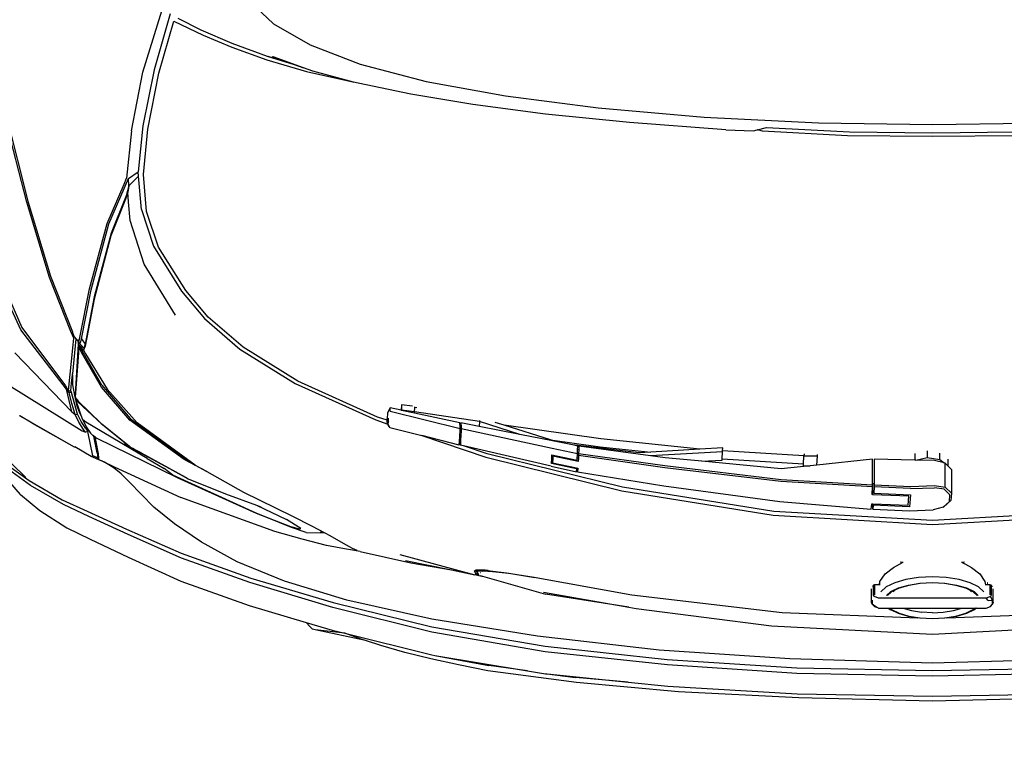
# Model space of a CAD drawing. Units: inches. Extents: x 1319 to 2030, y 219 to 1069.
# Tile 5 of 28: x 1434 to 1464, y 357 to 380. Entities that reach past the tile are written whole.
import ezdxf

# ---------------------------------------------------------------- set-up
doc = ezdxf.new("R2010")
doc.units = ezdxf.units.IN
doc.header["$MEASUREMENT"] = 0
doc.layers.get('0').update_dxf_attribs({"color": 12})
doc.layers.add('A-ANNO-DIMS', color=2, linetype='Continuous', lineweight=18)
doc.layers.add('C-PRKG-VEHC', color=8, linetype='Continuous', lineweight=13)
doc.layers.add('Edges', color=250, linetype='Continuous')
doc.styles.get("Standard").update_dxf_attribs({"font": 'arial.ttf'})
doc.dimstyles.get("Standard").update_dxf_attribs({"dimtxt": 7, "dimasz": 0.18, "dimexe": 0.18, "dimexo": 0.0625, "dimgap": 0.09, "dimtad": 0, "dimtih": 1, "dimtoh": 1, "dimzin": 0, "dimdsep": 46, "dimlunit": 3, "dimtxsty": 'Standard', "dimcen": 0.09, "dimadec": 0, "dimazin": 0, "dimtfac": 1, "dimtofl": 0, "dimtmove": 0, "dimatfit": 3, "dimfxl": 1, "dimtolj": 1, "dimtzin": 0, "dimarcsym": 0})

# ---------------------------------------------------------------- blocks, each defined once
blk = doc.blocks.new('Nissan Qashqai pl')
at = {"layer": 'Edges'}
for p, q in [((11.5166, 12.04708), (11.52386, 11.92208)), ((11.52698, 11.92208), (11.51964, 12.0475)), ((11.61327, 11.92208), (11.60675, 12.04892)), ((11.60051, 11.93346), (11.59629, 12.04057)), ((11.63292, 12.0344), (11.63628, 11.92208)), ((11.64211, 11.92208), (11.63993, 12.02899)), ((11.64437, 12.02886), (11.64655, 11.92208)), ((11.66226, 11.92208), (11.66041, 12.02874)), ((11.66349, 12.02738), (11.66628, 11.92208)), ((11.21164, 11.92208), (11.21014, 12.01197)), ((11.22044, 11.98904), (11.22108, 11.92208)), ((11.21801, 11.92208), (11.21745, 11.98742)), ((11.57261, 11.96533), (11.57261, 11.96561)), ((11.57306, 11.96528), (11.57306, 11.96569)), ((11.57479, 11.96843), (11.57457, 11.96768)), ((11.58239, 11.96768), (11.57457, 11.96768)), ((11.57457, 11.96768), (11.57457, 11.96395)), ((11.57617, 11.96938), (11.57479, 11.96843)), ((11.57479, 11.96843), (11.58262, 11.96843)), ((11.58846, 11.97008), (11.57758, 11.97008)), ((11.58262, 11.96843), (11.58377, 11.96782)), ((11.58668, 11.96947), (11.58377, 11.96782)), ((11.58377, 11.96782), (11.58513, 11.96453)), ((11.58679, 11.96604), (11.58513, 11.96453)), ((11.58679, 11.96604), (11.58668, 11.96947)), ((11.58961, 11.96947), (11.58668, 11.96947)), ((11.58846, 11.97008), (11.58961, 11.96947)), ((11.5915, 11.96782), (11.58961, 11.96947)), ((11.5915, 11.96782), (11.59043, 11.96839)), ((11.59285, 11.96453), (11.5915, 11.96782)), ((11.56082, 11.95281), (11.56588, 11.95938)), ((11.56588, 11.95938), (11.57195, 11.96347)), ((11.57195, 11.96347), (11.57457, 11.96395)), ((11.57613, 11.95845), (11.57286, 11.95178)), ((11.57457, 11.96395), (11.57457, 11.96378)), ((11.57994, 11.96265), (11.57613, 11.95845)), ((11.57987, 11.95487), (11.58291, 11.95821)), ((11.58513, 11.96453), (11.58513, 11.87963)), ((11.59285, 11.95694), (11.59285, 11.96453)), ((11.55816, 11.94815), (11.56082, 11.95281)), ((11.57286, 11.95178), (11.57035, 11.94308)), ((11.57692, 11.94885), (11.57987, 11.95487)), ((11.57876, 11.95169), (11.57712, 11.94834)), ((11.58001, 11.95424), (11.57876, 11.95169)), ((11.57876, 11.95169), (11.57995, 11.953)), ((11.58291, 11.95743), (11.58001, 11.95424)), ((11.59285, 11.95694), (11.59412, 11.95487)), ((11.59285, 11.95657), (11.59285, 11.95694)), ((11.59319, 11.9559), (11.59285, 11.95657)), ((11.59285, 11.95626), (11.59285, 11.95657)), ((11.59285, 11.95626), (11.59319, 11.9559)), ((11.59285, 11.95549), (11.59285, 11.95626)), ((11.59398, 11.95424), (11.59285, 11.95549)), ((11.59285, 11.94526), (11.59285, 11.95549)), ((11.59319, 11.9559), (11.59412, 11.95487)), ((11.59688, 11.94834), (11.59398, 11.95424)), ((11.59412, 11.95487), (11.59707, 11.94885)), ((11.55654, 11.94509), (11.55639, 11.94749)), ((11.55654, 11.94509), (11.55816, 11.94815)), ((11.57035, 11.94308), (11.56877, 11.93295)), ((11.57466, 11.94101), (11.57692, 11.94885)), ((11.57712, 11.94834), (11.5749, 11.94065)), ((11.59285, 11.8989), (11.59285, 11.94526)), ((11.59478, 11.93858), (11.59285, 11.94526)), ((11.5991, 11.94065), (11.59688, 11.94834)), ((11.59707, 11.94885), (11.59933, 11.94101)), ((11.48106, 11.93457), (11.47554, 11.93456)), ((11.48106, 11.93457), (11.4786, 11.93206)), ((11.48349, 11.93703), (11.48106, 11.93457)), ((11.48349, 11.93703), (11.50222, 11.93704)), ((11.49744, 11.93207), (11.50222, 11.93704)), ((11.50349, 11.93588), (11.49907, 11.93132)), ((11.50222, 11.93704), (11.50812, 11.93671)), ((11.50889, 11.93558), (11.50349, 11.93588)), ((11.50812, 11.93671), (11.51287, 11.9312)), ((11.50889, 11.93558), (11.51321, 11.93053)), ((11.57324, 11.93188), (11.57466, 11.94101)), ((11.5749, 11.94065), (11.5735, 11.93169)), ((11.59602, 11.93062), (11.59478, 11.93858)), ((11.60049, 11.93169), (11.5991, 11.94065)), ((11.59933, 11.94101), (11.60051, 11.93346)), ((11.47578, 11.92803), (11.47062, 11.92803)), ((11.47398, 11.91798), (11.47578, 11.92803)), ((11.47578, 11.92803), (11.4784, 11.93124)), ((11.4784, 11.93124), (11.47657, 11.92368)), ((11.4786, 11.93206), (11.4784, 11.93124)), ((11.49744, 11.93207), (11.4786, 11.93206)), ((11.49621, 11.92369), (11.49744, 11.93207)), ((11.49907, 11.93132), (11.49795, 11.92364)), ((11.51321, 11.93053), (11.51287, 11.9312)), ((11.51321, 11.93053), (11.51543, 11.92267)), ((11.56877, 11.93295), (11.56823, 11.92208)), ((11.57275, 11.92208), (11.57324, 11.93188)), ((11.5735, 11.93169), (11.57302, 11.92208)), ((11.59645, 11.92208), (11.59602, 11.93062)), ((11.60097, 11.92208), (11.60049, 11.93169)), ((11.60051, 11.93346), (11.60076, 11.93188)), ((11.60076, 11.93188), (11.60124, 11.92208)), ((11.21014, 11.8322), (11.21164, 11.92208)), ((11.21745, 11.85674), (11.21801, 11.92208)), ((11.22108, 11.92208), (11.22044, 11.85512)), ((11.47657, 11.92368), (11.47622, 11.90912)), ((11.49689, 11.90495), (11.49621, 11.92369)), ((11.49859, 11.9049), (11.49795, 11.92364)), ((11.51606, 11.90392), (11.51543, 11.92267)), ((11.52386, 11.92208), (11.5166, 11.79708)), ((11.51964, 11.79666), (11.52698, 11.92208)), ((11.56823, 11.92208), (11.56877, 11.91121)), ((11.57324, 11.91228), (11.57275, 11.92208)), ((11.57302, 11.92208), (11.5735, 11.91247)), ((11.59645, 11.92208), (11.59602, 11.91354)), ((11.60049, 11.91247), (11.60097, 11.92208)), ((11.60124, 11.92208), (11.60076, 11.91228)), ((11.60675, 11.79524), (11.61327, 11.92208)), ((11.63628, 11.92208), (11.63292, 11.80976)), ((11.63993, 11.81518), (11.64211, 11.92208)), ((11.64655, 11.92208), (11.64437, 11.8153)), ((11.66041, 11.81542), (11.66226, 11.92208)), ((11.66628, 11.92208), (11.66349, 11.81678)), ((11.46896, 11.91798), (11.47398, 11.91798)), ((11.47622, 11.90912), (11.47398, 11.91798)), ((11.56877, 11.91121), (11.57035, 11.90108)), ((11.57466, 11.90315), (11.57324, 11.91228)), ((11.5735, 11.91247), (11.5749, 11.90351)), ((11.59478, 11.90558), (11.59602, 11.91354)), ((11.5991, 11.90351), (11.60049, 11.91247)), ((11.60076, 11.91228), (11.60051, 11.91071)), ((11.47102, 11.90825), (11.4762, 11.90826)), ((11.4762, 11.90826), (11.47542, 11.87608)), ((11.47622, 11.90912), (11.4762, 11.90826)), ((11.49565, 11.87616), (11.49689, 11.90495)), ((11.49859, 11.9049), (11.49735, 11.87612)), ((11.50223, 11.8759), (11.50346, 11.90468)), ((11.50462, 11.90341), (11.50341, 11.87505)), ((11.50346, 11.90468), (11.51299, 11.90415)), ((11.51177, 11.90301), (11.50462, 11.90341)), ((11.51299, 11.90415), (11.51176, 11.87537)), ((11.51483, 11.87514), (11.51606, 11.90392)), ((11.5749, 11.90351), (11.57712, 11.89582)), ((11.59285, 11.8989), (11.59478, 11.90558)), ((11.59629, 11.80359), (11.60051, 11.91071)), ((11.59688, 11.89582), (11.5991, 11.90351)), ((11.60051, 11.91071), (11.59933, 11.90315)), ((11.51058, 11.87508), (11.51177, 11.90301)), ((11.55639, 11.89667), (11.55654, 11.89907)), ((11.55816, 11.89601), (11.55654, 11.89907)), ((11.56082, 11.89135), (11.55816, 11.89601)), ((11.57035, 11.90108), (11.57286, 11.89238)), ((11.57692, 11.89531), (11.57466, 11.90315)), ((11.57712, 11.89582), (11.57876, 11.89248)), ((11.59285, 11.88868), (11.59285, 11.8989)), ((11.59398, 11.88992), (11.59688, 11.89582)), ((11.59933, 11.90315), (11.59707, 11.89531)), ((11.56588, 11.88478), (11.56082, 11.89135)), ((11.57286, 11.89238), (11.57613, 11.88571)), ((11.57987, 11.88929), (11.57692, 11.89531)), ((11.57995, 11.89116), (11.57876, 11.89248)), ((11.57876, 11.89248), (11.58001, 11.88992)), ((11.58291, 11.88595), (11.57987, 11.88929)), ((11.58001, 11.88992), (11.58291, 11.88673)), ((11.59285, 11.88868), (11.59398, 11.88992)), ((11.59285, 11.88722), (11.59412, 11.88929)), ((11.59285, 11.8879), (11.59285, 11.88868)), ((11.59285, 11.88759), (11.59319, 11.88827)), ((11.59319, 11.88827), (11.59285, 11.8879)), ((11.59285, 11.88759), (11.59285, 11.8879)), ((11.59412, 11.88929), (11.59319, 11.88827)), ((11.59707, 11.89531), (11.59412, 11.88929)), ((11.57195, 11.88069), (11.56588, 11.88478)), ((11.57261, 11.88057), (11.57195, 11.88069)), ((11.57261, 11.88057), (11.57261, 11.88076)), ((11.57306, 11.88049), (11.57261, 11.88057)), ((11.57306, 11.88049), (11.57306, 11.88081)), ((11.57457, 11.88021), (11.57306, 11.88049)), ((11.57457, 11.88096), (11.57457, 11.88021)), ((11.57457, 11.88021), (11.57457, 11.87648)), ((11.57613, 11.88571), (11.57994, 11.88151)), ((11.59285, 11.88722), (11.59285, 11.88759)), ((11.59285, 11.87963), (11.59285, 11.88722)), ((11.49563, 11.87496), (11.47539, 11.87488)), ((11.47539, 11.87488), (11.4801, 11.83099)), ((11.47542, 11.87608), (11.49451, 11.87616)), ((11.49133, 11.80278), (11.49563, 11.87496)), ((11.49732, 11.87492), (11.49295, 11.80271)), ((11.49449, 11.87502), (11.49451, 11.87616)), ((11.50341, 11.87505), (11.49449, 11.87502)), ((11.49451, 11.87616), (11.49565, 11.87616)), ((11.49732, 11.87492), (11.49563, 11.87496)), ((11.49565, 11.87616), (11.49735, 11.87612)), ((11.50339, 11.87463), (11.49732, 11.87492)), ((11.49735, 11.87612), (11.50223, 11.8759)), ((11.50341, 11.87505), (11.50339, 11.87463)), ((11.50884, 11.80182), (11.5148, 11.87394)), ((11.51054, 11.87423), (11.51058, 11.87508)), ((11.5148, 11.87394), (11.51054, 11.87423)), ((11.51472, 11.8751), (11.51058, 11.87508)), ((11.51176, 11.87537), (11.51472, 11.87515)), ((11.51472, 11.87515), (11.51472, 11.8751)), ((11.51472, 11.87515), (11.51483, 11.87514)), ((11.51483, 11.87514), (11.51472, 11.8751)), ((11.57457, 11.87648), (11.58239, 11.87648)), ((11.57457, 11.87648), (11.57479, 11.87573)), ((11.58262, 11.87573), (11.57479, 11.87573)), ((11.57479, 11.87573), (11.57617, 11.87478)), ((11.58846, 11.87408), (11.57758, 11.87408)), ((11.58377, 11.87635), (11.58262, 11.87573)), ((11.58513, 11.87963), (11.58377, 11.87635)), ((11.58668, 11.87469), (11.58961, 11.87469)), ((11.58961, 11.87469), (11.58846, 11.87408)), ((11.58961, 11.87469), (11.5915, 11.87635)), ((11.59043, 11.87577), (11.58961, 11.87469)), ((11.59221, 11.87812), (11.59043, 11.87577)), ((11.59043, 11.87577), (11.5915, 11.87635)), ((11.5915, 11.87635), (11.59221, 11.87812)), ((11.59285, 11.87963), (11.59221, 11.87812)), ((11.2139, 11.7914), (11.21745, 11.85674)), ((11.22044, 11.85512), (11.21682, 11.78816)), ((11.20565, 11.74231), (11.21014, 11.8322)), ((11.47305, 11.83139), (11.47165, 11.83144)), ((11.47305, 11.83139), (11.473, 11.82087)), ((11.4801, 11.83099), (11.47305, 11.83139)), ((11.4801, 11.83099), (11.48065, 11.82584)), ((11.48062, 11.82044), (11.48065, 11.82584)), ((11.48065, 11.82584), (11.4831, 11.803)), ((11.47281, 11.82086), (11.46872, 11.75675)), ((11.47111, 11.82093), (11.47189, 11.82089)), ((11.47281, 11.82086), (11.47189, 11.82089)), ((11.473, 11.82087), (11.47281, 11.82086)), ((11.47916, 11.8205), (11.473, 11.82087)), ((11.47508, 11.75641), (11.47919, 11.82046)), ((11.47919, 11.82046), (11.47916, 11.8205)), ((11.48062, 11.82044), (11.47919, 11.82046)), ((11.63327, 11.71316), (11.63993, 11.81518)), ((11.64437, 11.8153), (11.63768, 11.7134)), ((11.65425, 11.71357), (11.66041, 11.81542)), ((11.66349, 11.81678), (11.65888, 11.72193)), ((11.4831, 11.803), (11.47707, 11.74042)), ((11.4805, 11.71128), (11.49133, 11.80278)), ((11.49295, 11.80271), (11.48212, 11.71121)), ((11.58235, 11.68521), (11.59629, 11.80359)), ((11.63292, 11.80976), (11.62604, 11.70665)), ((11.49642, 11.71041), (11.50884, 11.80182)), ((11.5166, 11.79708), (11.49761, 11.67796)), ((11.50045, 11.6772), (11.51964, 11.79666)), ((11.5932, 11.68852), (11.60675, 11.79524)), ((11.21579, 11.78424), (11.2139, 11.7914)), ((11.21682, 11.78816), (11.21579, 11.78424)), ((11.21682, 11.78816), (11.21585, 11.78401)), ((11.21585, 11.78401), (11.21579, 11.78424)), ((11.21658, 11.78121), (11.21585, 11.78401)), ((11.21586, 11.75915), (11.21658, 11.78121)), ((11.21586, 11.75915), (11.20997, 11.68347)), ((11.46872, 11.75675), (11.46649, 11.75682)), ((11.46649, 11.75682), (11.46757, 11.73891)), ((11.46975, 11.75671), (11.46872, 11.75675)), ((11.46975, 11.75671), (11.47273, 11.69994)), ((11.47508, 11.75641), (11.46975, 11.75671)), ((11.47611, 11.75636), (11.47508, 11.75641)), ((11.47707, 11.74042), (11.47611, 11.75636)), ((11.19842, 11.65867), (11.20565, 11.74231)), ((11.47707, 11.74042), (11.47428, 11.71144)), ((11.46757, 11.73891), (11.45941, 11.6607)), ((11.46757, 11.73891), (11.46992, 11.70014)), ((11.65888, 11.72193), (11.65143, 11.64152)), ((11.47094, 11.64327), (11.4805, 11.71128)), ((11.48212, 11.71121), (11.47257, 11.6432)), ((11.47428, 11.71144), (11.47273, 11.69994)), ((11.48539, 11.64249), (11.49642, 11.71041)), ((11.6229, 11.61679), (11.63327, 11.71316)), ((11.63768, 11.7134), (11.62719, 11.61693)), ((11.65114, 11.68233), (11.65425, 11.71357)), ((11.62604, 11.70665), (11.61495, 11.61084)), ((11.47273, 11.69994), (11.46512, 11.64343)), ((11.46576, 11.66035), (11.46992, 11.70014)), ((11.46992, 11.70014), (11.47047, 11.69095)), ((11.47047, 11.69095), (11.46419, 11.63849)), ((11.59218, 11.68277), (11.5932, 11.68852)), ((11.20997, 11.68347), (11.2033, 11.61723)), ((11.56846, 11.60829), (11.58235, 11.68521)), ((11.58021, 11.61555), (11.59218, 11.68277)), ((11.59218, 11.68277), (11.58179, 11.61717)), ((11.64478, 11.61839), (11.65114, 11.68233)), ((11.65114, 11.68233), (11.64749, 11.64092)), ((11.49761, 11.67796), (11.47115, 11.57128)), ((11.47375, 11.5702), (11.50045, 11.6772)), ((11.18907, 11.58559), (11.19842, 11.65867)), ((11.45941, 11.6607), (11.44866, 11.58459)), ((11.46024, 11.62121), (11.46576, 11.66035)), ((11.46505, 11.64255), (11.46419, 11.63849)), ((11.46792, 11.64248), (11.46505, 11.64255)), ((11.46512, 11.64343), (11.46801, 11.64335)), ((11.46687, 11.62247), (11.47088, 11.64239)), ((11.46801, 11.64335), (11.46792, 11.64248)), ((11.47088, 11.64239), (11.46792, 11.64248)), ((11.46801, 11.64335), (11.47094, 11.64327)), ((11.47252, 11.64233), (11.47088, 11.64239)), ((11.47094, 11.64327), (11.47257, 11.6432)), ((11.47212, 11.62223), (11.47625, 11.64214)), ((11.47439, 11.64223), (11.47252, 11.64233)), ((11.47257, 11.6432), (11.47449, 11.6431)), ((11.47727, 11.64296), (11.47315, 11.62305)), ((11.47439, 11.64223), (11.47449, 11.6431)), ((11.47625, 11.64214), (11.47439, 11.64223)), ((11.47449, 11.6431), (11.47727, 11.64296)), ((11.47827, 11.62277), (11.48226, 11.64167)), ((11.48298, 11.64165), (11.47879, 11.62186)), ((11.48098, 11.62171), (11.48532, 11.64161)), ((11.48226, 11.64167), (11.48244, 11.64254)), ((11.48226, 11.64167), (11.48298, 11.64165)), ((11.48244, 11.64254), (11.48247, 11.64267)), ((11.48535, 11.64246), (11.48244, 11.64254)), ((11.48247, 11.64267), (11.48535, 11.64246)), ((11.483, 11.64176), (11.48298, 11.64165)), ((11.48532, 11.64161), (11.483, 11.64176)), ((11.48539, 11.64249), (11.48535, 11.64246)), ((11.65143, 11.64152), (11.64217, 11.57162)), ((11.64478, 11.61839), (11.64749, 11.64092)), ((11.46419, 11.63849), (11.46114, 11.62406)), ((11.46114, 11.62406), (11.46024, 11.62121)), ((11.46114, 11.62406), (11.46083, 11.62261)), ((11.2033, 11.61723), (11.19582, 11.55976)), ((11.46024, 11.62121), (11.44866, 11.58459)), ((11.45125, 11.55073), (11.46687, 11.62247)), ((11.46083, 11.62261), (11.45585, 11.5969)), ((11.48098, 11.62171), (11.4649, 11.55261)), ((11.47495, 11.62207), (11.47212, 11.62223)), ((11.47315, 11.62305), (11.47515, 11.62294)), ((11.47495, 11.62207), (11.47515, 11.62294)), ((11.47879, 11.62186), (11.47495, 11.62207)), ((11.47515, 11.62294), (11.47827, 11.62277)), ((11.56776, 11.56755), (11.58179, 11.61717)), ((11.60765, 11.5276), (11.6229, 11.61679)), ((11.62719, 11.61693), (11.61178, 11.52762)), ((11.64227, 11.603), (11.64462, 11.61709)), ((11.64462, 11.61709), (11.64478, 11.61839)), ((11.56905, 11.60888), (11.56563, 11.58822)), ((11.61495, 11.61084), (11.6016, 11.52761)), ((11.56499, 11.58644), (11.56846, 11.60829)), ((11.63012, 11.53004), (11.64227, 11.603)), ((11.64227, 11.603), (11.63807, 11.5726)), ((11.45585, 11.5969), (11.44582, 11.56516)), ((11.45585, 11.5969), (11.44965, 11.56495)), ((11.17758, 11.52307), (11.18907, 11.58559)), ((11.56356, 11.57357), (11.56499, 11.58644)), ((11.56563, 11.58822), (11.56415, 11.57536)), ((11.44723, 11.58007), (11.44639, 11.57739)), ((11.44866, 11.58459), (11.44723, 11.58007)), ((11.45676, 11.51971), (11.47375, 11.5702)), ((11.47115, 11.57128), (11.4649, 11.55261)), ((11.56268, 11.56956), (11.56259, 11.5697)), ((11.56268, 11.56956), (11.5628, 11.57206)), ((11.56335, 11.56843), (11.56356, 11.57357)), ((11.56415, 11.57536), (11.56375, 11.56794)), ((11.63012, 11.53004), (11.63807, 11.5726)), ((11.64217, 11.57162), (11.63751, 11.54857)), ((11.44575, 11.56516), (11.43801, 11.51398)), ((11.4448, 11.5652), (11.44575, 11.56516)), ((11.44575, 11.56516), (11.44582, 11.56516)), ((11.44582, 11.56516), (11.44965, 11.56495)), ((11.44965, 11.56495), (11.44685, 11.5505)), ((11.56255, 11.56701), (11.56268, 11.56956)), ((11.56271, 11.56245), (11.56255, 11.56701)), ((11.56335, 11.56843), (11.56268, 11.56956)), ((11.56334, 11.56271), (11.56271, 11.56245)), ((11.56338, 11.56129), (11.56271, 11.56245)), ((11.56325, 11.56586), (11.56335, 11.56843)), ((11.56334, 11.56271), (11.56325, 11.56586)), ((11.56609, 11.56386), (11.56334, 11.56271)), ((11.56338, 11.56129), (11.56334, 11.56271)), ((11.56368, 11.56788), (11.56335, 11.56843)), ((11.56583, 11.56223), (11.56338, 11.56129)), ((11.56375, 11.56794), (11.56392, 11.56325)), ((11.56392, 11.56325), (11.56429, 11.56338)), ((11.56429, 11.56338), (11.56596, 11.56408)), ((11.56487, 11.5659), (11.56469, 11.5662)), ((11.56609, 11.56386), (11.56583, 11.56223)), ((11.56616, 11.56236), (11.56583, 11.56223)), ((11.56596, 11.56408), (11.56616, 11.56417)), ((11.56609, 11.56386), (11.56596, 11.56408)), ((11.56613, 11.56388), (11.56609, 11.56386)), ((11.56618, 11.56418), (11.56613, 11.56388)), ((11.56613, 11.56388), (11.56616, 11.56417)), ((11.56613, 11.56388), (11.56645, 11.5641)), ((11.56665, 11.56424), (11.56616, 11.56236)), ((11.56616, 11.56417), (11.56618, 11.56418)), ((11.56616, 11.56236), (11.56645, 11.5641)), ((11.56661, 11.56253), (11.56616, 11.56236)), ((11.56618, 11.56418), (11.56648, 11.56431)), ((11.56645, 11.5641), (11.56648, 11.56431)), ((11.56645, 11.5641), (11.56665, 11.56424)), ((11.56648, 11.56431), (11.56669, 11.5644)), ((11.56679, 11.56261), (11.56648, 11.56144)), ((11.56661, 11.56253), (11.56704, 11.56455)), ((11.56671, 11.56257), (11.56661, 11.56253)), ((11.56665, 11.56424), (11.56688, 11.56448)), ((11.56669, 11.5644), (11.56665, 11.56424)), ((11.56669, 11.5644), (11.56688, 11.56448)), ((11.56671, 11.56257), (11.56712, 11.56458)), ((11.56679, 11.56261), (11.56671, 11.56257)), ((11.56717, 11.5646), (11.56679, 11.56261)), ((11.56688, 11.56448), (11.56704, 11.56455)), ((11.56704, 11.56455), (11.56739, 11.56625)), ((11.56704, 11.56455), (11.56712, 11.56458)), ((11.56712, 11.56458), (11.56763, 11.56708)), ((11.56712, 11.56458), (11.56717, 11.5646)), ((11.56717, 11.5646), (11.56763, 11.56708)), ((11.56745, 11.56646), (11.56739, 11.56625)), ((11.56763, 11.56708), (11.56776, 11.56755)), ((11.19582, 11.55976), (11.18773, 11.51111)), ((11.55053, 11.5023), (11.56648, 11.56144)), ((11.56273, 11.5431), (11.56648, 11.56144)), ((11.43747, 11.49463), (11.45125, 11.54985)), ((11.44684, 11.54963), (11.43914, 11.51392)), ((11.44983, 11.54978), (11.44684, 11.54963)), ((11.44685, 11.5505), (11.44997, 11.55066)), ((11.44983, 11.54978), (11.44997, 11.55066)), ((11.45125, 11.54985), (11.44983, 11.54978)), ((11.44997, 11.55066), (11.45125, 11.55073)), ((11.45125, 11.55073), (11.4529, 11.55066)), ((11.4529, 11.54978), (11.45125, 11.54985)), ((11.4529, 11.55066), (11.45711, 11.55045)), ((11.45711, 11.54958), (11.4529, 11.54978)), ((11.46429, 11.54915), (11.45676, 11.51971)), ((11.45711, 11.55045), (11.45994, 11.5503)), ((11.46197, 11.5493), (11.45711, 11.54958)), ((11.45983, 11.54978), (11.45994, 11.5503)), ((11.46402, 11.54999), (11.45983, 11.54978)), ((11.45994, 11.5503), (11.46197, 11.55018)), ((11.46197, 11.55018), (11.46404, 11.55004)), ((11.46375, 11.54918), (11.46197, 11.5493)), ((11.46402, 11.54999), (11.46375, 11.54918)), ((11.46429, 11.54915), (11.46375, 11.54918)), ((11.46404, 11.55004), (11.46402, 11.54999)), ((11.46423, 11.55), (11.46402, 11.54999)), ((11.46404, 11.55004), (11.46423, 11.55)), ((11.46423, 11.55), (11.46424, 11.55003)), ((11.4643, 11.55002), (11.46423, 11.55)), ((11.4649, 11.55261), (11.4643, 11.55002)), ((11.63751, 11.54857), (11.63276, 11.52672)), ((11.55533, 11.50682), (11.56273, 11.5431)), ((11.55707, 11.51104), (11.56273, 11.5431)), ((11.16395, 11.47112), (11.17758, 11.52307)), ((11.6016, 11.52761), (11.58664, 11.46068)), ((11.58843, 11.44985), (11.60765, 11.5276)), ((11.61178, 11.52762), (11.59225, 11.44945)), ((11.61272, 11.45895), (11.62966, 11.52759)), ((11.63276, 11.52672), (11.62771, 11.50627)), ((11.62966, 11.52759), (11.63012, 11.53004)), ((11.43501, 11.51584), (11.43475, 11.51409)), ((11.45032, 11.49453), (11.45676, 11.51971)), ((11.18773, 11.51111), (11.17906, 11.46956)), ((11.43371, 11.51238), (11.43251, 11.50378)), ((11.43475, 11.51409), (11.43403, 11.51411)), ((11.43801, 11.51398), (11.43475, 11.51409)), ((11.4382, 11.51397), (11.43676, 11.50364)), ((11.43914, 11.51392), (11.43692, 11.50363)), ((11.4382, 11.51397), (11.43801, 11.51398)), ((11.43914, 11.51392), (11.4382, 11.51397)), ((11.54814, 11.47101), (11.55707, 11.51104)), ((11.43251, 11.50378), (11.43676, 11.50364)), ((11.43251, 11.50378), (11.4369, 11.50353)), ((11.4369, 11.50353), (11.435, 11.49469)), ((11.43676, 11.50364), (11.43692, 11.50363)), ((11.43692, 11.50363), (11.4369, 11.50353)), ((11.62771, 11.50627), (11.62241, 11.48743)), ((11.435, 11.49469), (11.43896, 11.49272)), ((11.43747, 11.49463), (11.435, 11.49469)), ((11.43896, 11.49272), (11.44373, 11.49245)), ((11.44474, 11.49242), (11.44218, 11.48476)), ((11.44507, 11.49341), (11.44316, 11.49351)), ((11.44373, 11.49245), (11.44491, 11.49291)), ((11.44474, 11.49242), (11.44373, 11.49245)), ((11.44453, 11.48334), (11.44778, 11.49299)), ((11.44491, 11.49291), (11.44474, 11.49242)), ((11.4462, 11.49239), (11.44474, 11.49242)), ((11.44507, 11.49341), (11.44491, 11.49291)), ((11.44491, 11.49291), (11.44606, 11.49335)), ((11.44606, 11.49335), (11.44507, 11.49341)), ((11.44786, 11.49325), (11.44606, 11.49335)), ((11.44786, 11.49325), (11.4462, 11.49239)), ((11.44778, 11.49299), (11.4462, 11.49239)), ((11.45018, 11.49392), (11.44778, 11.49299)), ((11.44794, 11.49325), (11.44786, 11.49325)), ((11.45032, 11.49453), (11.44794, 11.49325)), ((11.45018, 11.49392), (11.45032, 11.49453)), ((11.44218, 11.48476), (11.41383, 11.42186)), ((11.62241, 11.48743), (11.61848, 11.47528)), ((11.41588, 11.41997), (11.44453, 11.48334)), ((11.14869, 11.43161), (11.16395, 11.47112)), ((11.17906, 11.46956), (11.17808, 11.46592)), ((11.54814, 11.47101), (11.54666, 11.46197)), ((11.61848, 11.47528), (11.61008, 11.43562)), ((11.61742, 11.47198), (11.61272, 11.45895)), ((11.61848, 11.47528), (11.61742, 11.47198)), ((11.17808, 11.46592), (11.1694, 11.43374)), ((11.1699, 11.42889), (11.17797, 11.4652)), ((11.17797, 11.4652), (11.17808, 11.46592)), ((11.54162, 11.45783), (11.54554, 11.46484)), ((11.54554, 11.46484), (11.54721, 11.46841)), ((11.54666, 11.46197), (11.54611, 11.45874)), ((11.53572, 11.44731), (11.54162, 11.45783)), ((11.54611, 11.45874), (11.54336, 11.44449)), ((11.58664, 11.46068), (11.57152, 11.41151)), ((11.61272, 11.45895), (11.61008, 11.43562)), ((11.61028, 11.44915), (11.61272, 11.45895)), ((11.53354, 11.44315), (11.53572, 11.44731)), ((11.56912, 11.38501), (11.58843, 11.44985)), ((11.59225, 11.44945), (11.57263, 11.38419)), ((11.60419, 11.42861), (11.61028, 11.44915)), ((11.52833, 11.43321), (11.53335, 11.4428)), ((11.53261, 11.43965), (11.5333, 11.44225)), ((11.53313, 11.42848), (11.53354, 11.44315)), ((11.5333, 11.44225), (11.53335, 11.4428)), ((11.53335, 11.4428), (11.53354, 11.44315)), ((11.54336, 11.44449), (11.53855, 11.42543)), ((11.1323, 11.40268), (11.14869, 11.43161)), ((11.1694, 11.43374), (11.1668, 11.42651)), ((11.5202, 11.41712), (11.52833, 11.43321)), ((11.60772, 11.43162), (11.60419, 11.42861)), ((11.60938, 11.43347), (11.60772, 11.43162)), ((11.61008, 11.43562), (11.60938, 11.43347)), ((11.1668, 11.42651), (11.1582, 11.40259)), ((11.16047, 11.39766), (11.1699, 11.42889)), ((11.16426, 11.41918), (11.1668, 11.42651)), ((11.53009, 11.42439), (11.52299, 11.41307)), ((11.52855, 11.41625), (11.53022, 11.42324)), ((11.53313, 11.42848), (11.52922, 11.417)), ((11.53022, 11.42324), (11.53009, 11.42439)), ((11.53855, 11.42543), (11.53253, 11.4038)), ((11.59084, 11.38361), (11.60419, 11.42861)), ((11.15764, 11.39828), (11.16426, 11.41918)), ((11.15766, 11.39771), (11.16426, 11.41918)), ((11.16426, 11.41918), (11.15826, 11.40186)), ((11.41383, 11.42186), (11.38718, 11.37878)), ((11.38877, 11.37638), (11.41588, 11.41997)), ((11.50131, 11.37908), (11.5202, 11.41712)), ((11.52922, 11.417), (11.51787, 11.38901)), ((11.51787, 11.38901), (11.52855, 11.41625)), ((11.5118, 11.38938), (11.52299, 11.41307)), ((11.57152, 11.41151), (11.55624, 11.37411)), ((11.11477, 11.38434), (11.1323, 11.40268)), ((11.53253, 11.4038), (11.50574, 11.32965)), ((11.14751, 11.37001), (11.15766, 11.39771)), ((11.15051, 11.36998), (11.16047, 11.39766)), ((11.5118, 11.38938), (11.51304, 11.39274)), ((11.51787, 11.38901), (11.48801, 11.32337)), ((11.49005, 11.3275), (11.51787, 11.38901)), ((11.50277, 11.36495), (11.5118, 11.38938)), ((11.54963, 11.33002), (11.56912, 11.38501)), ((11.57263, 11.38419), (11.5535, 11.33028)), ((11.57164, 11.32969), (11.59084, 11.38361)), ((11.38718, 11.37878), (11.3635, 11.35125)), ((11.36451, 11.34835), (11.38877, 11.37638)), ((11.48518, 11.35017), (11.50131, 11.37908)), ((11.13692, 11.34555), (11.14751, 11.37001)), ((11.14123, 11.34726), (11.15051, 11.36998)), ((11.55624, 11.37411), (11.54097, 11.34593)), ((11.49086, 11.33567), (11.50277, 11.36495)), ((11.12767, 11.32749), (11.13692, 11.34555)), ((11.13017, 11.32416), (11.14123, 11.34726)), ((11.3635, 11.35125), (11.34251, 11.3336)), ((11.34283, 11.33026), (11.36451, 11.34835)), ((11.48518, 11.35017), (11.4758, 11.33232)), ((11.48012, 11.34111), (11.48518, 11.35017)), ((11.54097, 11.34593), (11.52646, 11.32473)), ((11.48005, 11.341), (11.44669, 11.29536)), ((11.47876, 11.33901), (11.47454, 11.33252)), ((11.47876, 11.33901), (11.48005, 11.341)), ((11.48005, 11.341), (11.48012, 11.34111)), ((11.30757, 11.30833), (11.34283, 11.33026)), ((11.34251, 11.3336), (11.3082, 11.31215)), ((11.44331, 11.28988), (11.47454, 11.33252)), ((11.4758, 11.33232), (11.44474, 11.28965)), ((11.46332, 11.28473), (11.48966, 11.33337)), ((11.47038, 11.29841), (11.49086, 11.33567)), ((11.47038, 11.29841), (11.48966, 11.33337)), ((11.48133, 11.27727), (11.50574, 11.32965)), ((11.48966, 11.33337), (11.49086, 11.33567)), ((11.53062, 11.28691), (11.54963, 11.33002)), ((11.5535, 11.33028), (11.53487, 11.28826)), ((11.55274, 11.28821), (11.57164, 11.32969)), ((11.1244, 11.32146), (11.16836, 11.30873)), ((11.17121, 11.31245), (11.13017, 11.32416)), ((11.36192, 11.32544), (11.32179, 11.30083)), ((11.45883, 11.26345), (11.48954, 11.32636)), ((11.48801, 11.32337), (11.48281, 11.31653)), ((11.48983, 11.32694), (11.48954, 11.32636)), ((11.48983, 11.32694), (11.49005, 11.3275)), ((11.52646, 11.32473), (11.51313, 11.30854)), ((11.17021, 11.29978), (11.11439, 11.31711)), ((11.47499, 11.30324), (11.48281, 11.31653)), ((11.16836, 11.30873), (11.21271, 11.29983)), ((11.21523, 11.3038), (11.17121, 11.31245)), ((11.27848, 11.29865), (11.30757, 11.30833)), ((11.3082, 11.31215), (11.28005, 11.30276)), ((11.51313, 11.30854), (11.49329, 11.28912)), ((11.21656, 11.2908), (11.17021, 11.29978)), ((11.21271, 11.29983), (11.24875, 11.29618)), ((11.2509, 11.3003), (11.21523, 11.3038)), ((11.28005, 11.30276), (11.2509, 11.3003)), ((11.27848, 11.29865), (11.25238, 11.29648)), ((11.32179, 11.30083), (11.28736, 11.28974)), ((11.47499, 11.30324), (11.4462, 11.25482)), ((11.46746, 11.29312), (11.47026, 11.29821)), ((11.47026, 11.29821), (11.47038, 11.29841)), ((11.21656, 11.2908), (11.25377, 11.28706)), ((11.25238, 11.29648), (11.24875, 11.29618)), ((11.2541, 11.28846), (11.24875, 11.29618)), ((11.25238, 11.29648), (11.25993, 11.28891)), ((11.42028, 11.27173), (11.44669, 11.29536)), ((11.46587, 11.29022), (11.46737, 11.29293)), ((11.46746, 11.29312), (11.46737, 11.29293)), ((11.25857, 11.28503), (11.25377, 11.28706)), ((11.25993, 11.28891), (11.2541, 11.28846)), ((11.29, 11.2731), (11.2541, 11.28846)), ((11.28951, 11.27177), (11.25857, 11.28503)), ((11.25993, 11.28891), (11.25999, 11.28889)), ((11.25999, 11.28889), (11.26503, 11.28789)), ((11.25999, 11.28889), (11.26771, 11.28668)), ((11.27242, 11.28847), (11.26503, 11.28789)), ((11.26503, 11.28789), (11.27055, 11.28622)), ((11.26771, 11.28668), (11.26785, 11.28663)), ((11.26785, 11.28663), (11.29721, 11.27493)), ((11.27055, 11.28622), (11.29928, 11.27468)), ((11.28736, 11.28974), (11.27242, 11.28847)), ((11.41708, 11.26758), (11.44331, 11.28988)), ((11.44474, 11.28965), (11.41866, 11.26734)), ((11.44691, 11.26684), (11.46587, 11.29022)), ((11.46538, 11.28932), (11.44788, 11.2676)), ((11.46538, 11.28932), (11.46587, 11.29022)), ((11.48692, 11.28262), (11.48256, 11.27724)), ((11.49329, 11.28912), (11.48692, 11.28262)), ((11.51652, 11.25601), (11.53062, 11.28691)), ((11.53487, 11.28826), (11.52058, 11.25724)), ((11.53843, 11.2583), (11.55274, 11.28821)), ((11.29721, 11.27493), (11.34742, 11.26142)), ((11.47707, 11.26812), (11.48133, 11.27727)), ((11.48256, 11.27724), (11.47783, 11.26953)), ((11.48133, 11.27727), (11.48217, 11.27864)), ((11.3411, 11.25789), (11.28951, 11.27177)), ((11.34188, 11.25916), (11.29, 11.2731)), ((11.29928, 11.27468), (11.34932, 11.2614)), ((11.41708, 11.26758), (11.38507, 11.24911)), ((11.41866, 11.26734), (11.3914, 11.25156)), ((11.39234, 11.25471), (11.42028, 11.27173)), ((11.44788, 11.2676), (11.43028, 11.24852)), ((11.47783, 11.26953), (11.47588, 11.26517)), ((11.47707, 11.26812), (11.47588, 11.26517)), ((11.34742, 11.26142), (11.38475, 11.2543)), ((11.34932, 11.2614), (11.38634, 11.25437)), ((11.42958, 11.2488), (11.44691, 11.26684)), ((11.47278, 11.2604), (11.45351, 11.25651)), ((11.45491, 11.25868), (11.45678, 11.26054)), ((11.4564, 11.26086), (11.45669, 11.26088)), ((11.45652, 11.26104), (11.45688, 11.26111)), ((11.45678, 11.26054), (11.45714, 11.2609)), ((11.45714, 11.2609), (11.45732, 11.2612)), ((11.45729, 11.26188), (11.45734, 11.2619)), ((11.47041, 11.26385), (11.45732, 11.2612)), ((11.45732, 11.2612), (11.45781, 11.262)), ((11.45736, 11.26195), (11.45734, 11.2619)), ((11.45736, 11.26195), (11.45755, 11.26195)), ((11.45781, 11.262), (11.45883, 11.26345)), ((11.45781, 11.262), (11.46047, 11.26254)), ((11.46047, 11.26254), (11.46049, 11.26254)), ((11.46049, 11.26254), (11.47129, 11.26473)), ((11.47322, 11.2592), (11.46579, 11.24614)), ((11.47041, 11.26385), (11.47423, 11.26446)), ((11.47129, 11.26473), (11.47442, 11.26498)), ((11.47269, 11.26007), (11.47281, 11.2603)), ((11.47463, 11.26457), (11.47278, 11.2604)), ((11.47423, 11.26446), (11.47278, 11.2604)), ((11.47278, 11.2604), (11.47281, 11.2603)), ((11.47281, 11.2603), (11.47317, 11.26096)), ((11.47281, 11.2603), (11.47322, 11.2592)), ((11.47585, 11.26509), (11.47322, 11.2592)), ((11.47423, 11.26446), (11.47445, 11.26449)), ((11.47442, 11.26498), (11.47433, 11.26475)), ((11.47442, 11.26498), (11.47446, 11.26498)), ((11.47445, 11.26477), (11.47446, 11.26498)), ((11.47463, 11.26457), (11.47445, 11.26449)), ((11.47446, 11.26498), (11.47482, 11.26501)), ((11.47585, 11.26509), (11.47463, 11.26457)), ((11.47482, 11.26501), (11.47475, 11.26484)), ((11.47482, 11.26501), (11.47585, 11.26509)), ((11.47588, 11.26517), (11.47585, 11.26509)), ((11.37955, 11.25028), (11.3411, 11.25789)), ((11.38043, 11.25154), (11.34188, 11.25916)), ((11.38043, 11.25154), (11.38475, 11.2543)), ((11.38408, 11.25081), (11.38043, 11.25154)), ((11.38295, 11.24897), (11.38801, 11.25321)), ((11.38475, 11.2543), (11.38801, 11.25321)), ((11.38823, 11.2519), (11.38491, 11.2491)), ((11.38811, 11.25194), (11.3861, 11.25078)), ((11.38634, 11.25437), (11.38953, 11.25299)), ((11.3914, 11.25156), (11.3867, 11.24922)), ((11.38862, 11.25223), (11.38822, 11.252)), ((11.38862, 11.25223), (11.38823, 11.2519)), ((11.39063, 11.25338), (11.38862, 11.25223)), ((11.38953, 11.25299), (11.38862, 11.25223)), ((11.38953, 11.25299), (11.39234, 11.25471)), ((11.41698, 11.19425), (11.45295, 11.25195)), ((11.44061, 11.25095), (11.44418, 11.2522)), ((11.44418, 11.2522), (11.44968, 11.25519)), ((11.4462, 11.25482), (11.44418, 11.2522)), ((11.45121, 11.25489), (11.44573, 11.25131)), ((11.45199, 11.25317), (11.44624, 11.24948)), ((11.44968, 11.25519), (11.44984, 11.25529)), ((11.44984, 11.25529), (11.45491, 11.25868)), ((11.44984, 11.25529), (11.45351, 11.25651)), ((11.45121, 11.25489), (11.45351, 11.25651)), ((11.45386, 11.25448), (11.45199, 11.25317)), ((11.45295, 11.25195), (11.45421, 11.25473)), ((11.45316, 11.25595), (11.45351, 11.25651)), ((11.45351, 11.25651), (11.45421, 11.25473)), ((11.45421, 11.25473), (11.45386, 11.25448)), ((11.47197, 11.25711), (11.47177, 11.25676)), ((11.50736, 11.23616), (11.51652, 11.25601)), ((11.52058, 11.25724), (11.51126, 11.23721)), ((11.52949, 11.24004), (11.53843, 11.2583)), ((11.33108, 11.22699), (11.37506, 11.24429)), ((11.38, 11.24532), (11.37475, 11.24309)), ((11.37506, 11.24429), (11.37524, 11.24436)), ((11.37506, 11.24429), (11.37621, 11.24429)), ((11.37922, 11.24593), (11.37524, 11.24436)), ((11.3763, 11.24436), (11.37524, 11.24436)), ((11.37922, 11.24593), (11.38041, 11.24692)), ((11.37933, 11.24631), (11.37922, 11.24593)), ((11.38338, 11.24949), (11.37955, 11.25028)), ((11.38533, 11.24487), (11.38, 11.24532)), ((11.38041, 11.24692), (11.38275, 11.24887)), ((11.38041, 11.24692), (11.40818, 11.24436)), ((11.38129, 11.24847), (11.38167, 11.2488)), ((11.38275, 11.24887), (11.38338, 11.24949)), ((11.38446, 11.24984), (11.38295, 11.24897)), ((11.38295, 11.24897), (11.38491, 11.2491)), ((11.38295, 11.24897), (11.38461, 11.24885)), ((11.38408, 11.25081), (11.38338, 11.24949)), ((11.38461, 11.24885), (11.38464, 11.24887)), ((11.38461, 11.24885), (11.38934, 11.2486)), ((11.38464, 11.24887), (11.38501, 11.24911)), ((11.38491, 11.2491), (11.38464, 11.24887)), ((11.38501, 11.24911), (11.38507, 11.24911)), ((11.38507, 11.24911), (11.3867, 11.24922)), ((11.42115, 11.24117), (11.38533, 11.24487)), ((11.3867, 11.24922), (11.3915, 11.24906)), ((11.38934, 11.2486), (11.42481, 11.24653)), ((11.3915, 11.24906), (11.42659, 11.2465)), ((11.3915, 11.19885), (11.4381, 11.24397)), ((11.41644, 11.24436), (11.40818, 11.24436)), ((11.40898, 11.24429), (11.40818, 11.24436)), ((11.40898, 11.24429), (11.4163, 11.24429)), ((11.4152, 11.24371), (11.40898, 11.24429)), ((11.4163, 11.24429), (11.4152, 11.24371)), ((11.42154, 11.24313), (11.4152, 11.24371)), ((11.41644, 11.24436), (11.4163, 11.24429)), ((11.41686, 11.24458), (11.41644, 11.24436)), ((11.4252, 11.2462), (11.41686, 11.24458)), ((11.43154, 11.24397), (11.42287, 11.24164)), ((11.43996, 11.24823), (11.42296, 11.24352)), ((11.42481, 11.24653), (11.42659, 11.2465)), ((11.42659, 11.2465), (11.4252, 11.2462)), ((11.42659, 11.2465), (11.42684, 11.24649)), ((11.42684, 11.24649), (11.42958, 11.2488)), ((11.42684, 11.24649), (11.42784, 11.24647)), ((11.43028, 11.24852), (11.42784, 11.24647)), ((11.42784, 11.24647), (11.42996, 11.24721)), ((11.4381, 11.24397), (11.42915, 11.24177)), ((11.42996, 11.24721), (11.43609, 11.24937)), ((11.43368, 11.248), (11.42996, 11.24721)), ((11.44027, 11.24637), (11.43154, 11.24397)), ((11.4397, 11.25049), (11.43368, 11.248)), ((11.43609, 11.24937), (11.44061, 11.25095)), ((11.4381, 11.24397), (11.44027, 11.24637)), ((11.44061, 11.25095), (11.4397, 11.25049)), ((11.44573, 11.25131), (11.43996, 11.24823)), ((11.44027, 11.24637), (11.43996, 11.24823)), ((11.44624, 11.24948), (11.44027, 11.24637)), ((11.44114, 11.20281), (11.46562, 11.24583)), ((11.44697, 11.21272), (11.46562, 11.24583)), ((11.46562, 11.24583), (11.46579, 11.24614)), ((11.37475, 11.24309), (11.33228, 11.22637)), ((11.3715, 11.20434), (11.41772, 11.23895)), ((11.42033, 11.23975), (11.37334, 11.20375)), ((11.41772, 11.23895), (11.41931, 11.23998)), ((11.41915, 11.23969), (11.4194, 11.23996)), ((11.41931, 11.23998), (11.4196, 11.24017)), ((11.4194, 11.23996), (11.41931, 11.23998)), ((11.4194, 11.23996), (11.4196, 11.24017)), ((11.41958, 11.23992), (11.4194, 11.23996)), ((11.4196, 11.24017), (11.42014, 11.24052)), ((11.41984, 11.24006), (11.42014, 11.24052)), ((11.42014, 11.24052), (11.42115, 11.24117)), ((11.42915, 11.24177), (11.42033, 11.23975)), ((11.42287, 11.24164), (11.42033, 11.23975)), ((11.42115, 11.24117), (11.42154, 11.24313)), ((11.42178, 11.24134), (11.42115, 11.24117)), ((11.42296, 11.24352), (11.42154, 11.24313)), ((11.42287, 11.24164), (11.42178, 11.24134)), ((11.42216, 11.24127), (11.42178, 11.24134)), ((11.42296, 11.24352), (11.42287, 11.24164)), ((11.49236, 11.21027), (11.50736, 11.23616)), ((11.51126, 11.23721), (11.49628, 11.21137)), ((11.51576, 11.21859), (11.52949, 11.24004)), ((11.27199, 11.20923), (11.33108, 11.22699)), ((11.33228, 11.22637), (11.27276, 11.20843)), ((11.44697, 11.21272), (11.44114, 11.20281)), ((11.50327, 11.20341), (11.51576, 11.21859)), ((11.20627, 11.19262), (11.27199, 11.20923)), ((11.27276, 11.20843), (11.20665, 11.19145)), ((11.45306, 11.16974), (11.48975, 11.20767)), ((11.47745, 11.18983), (11.49236, 11.21027)), ((11.49628, 11.21137), (11.48154, 11.19102)), ((11.31316, 11.17892), (11.3715, 11.20434)), ((11.37334, 11.20375), (11.31527, 11.17691)), ((11.44114, 11.20281), (11.4411, 11.20277)), ((11.50327, 11.20341), (11.49363, 11.19502))]:
    blk.add_line(p, q, dxfattribs=at)
blk = doc.blocks.new('car')
blk.add_blockref('Nissan Qashqai pl', (-9.74328, -11.91512))
blk = doc.blocks.new('carr')
blk.add_blockref('car', (0.51244, -0.00696))
blk = doc.blocks.new('*D57')
at = {"layer": 'A-ANNO-DIMS', "color": 0, "lineweight": -2, "transparency": 16777216}
for p, q in [((1419.914, 358.675), (1419.914, 332.688)), ((1504.443, 358.675), (1504.443, 332.688)), ((1420.094, 332.868), (1444.658, 332.868)), ((1504.263, 332.868), (1479.699, 332.868))]:
    blk.add_line(p, q, dxfattribs=at)
at = {"layer": 'A-ANNO-DIMS', "color": 0, "transparency": 16777216}
for points in [[(1420.094, 332.898), (1420.094, 332.838), (1419.914, 332.868)], [(1504.263, 332.898), (1504.263, 332.838), (1504.443, 332.868)]]:
    blk.add_solid(points, dxfattribs=at)
at = {"layer": 'Defpoints', "color": 0, "transparency": 16777216}
for p in [(1419.914, 358.738), (1504.443, 358.738), (1504.443, 332.868)]:
    blk.add_point(p, dxfattribs=at)
at = {"layer": 'A-ANNO-DIMS', "color": 0, "transparency": 16777216, "insert": (1462.179, 332.868), "char_height": 7, "attachment_point": 5}
blk.add_mtext('\\A1;7\'-0 1/2"', dxfattribs=at)

msp = doc.modelspace()

# ---------------------------------------------------------------- block references
at = {"layer": 'C-PRKG-VEHC', "xscale": 39.37007874015748, "yscale": 39.37007874015748, "zscale": 39.37007874015748, "rotation": 270}
msp.add_blockref('carr', (1462.179, 454.621), dxfattribs=at)

# ---------------------------------------------------------------- dimensions: what is measured, and where the dimension line sits
at = {"layer": 'A-ANNO-DIMS'}
dim = msp.add_linear_dim(base=(1504.443, 332.868), p1=(1419.914, 358.738), p2=(1504.443, 358.738), dimstyle='Standard', override={"dimdec": 1, "dimlfac": 1, "dimrnd": 0, "dimzin": 1, "dimdsep": 46, "dimlunit": 4, "dimfrac": 2}, dxfattribs=at)
dim.commit()
dim.dimension.update_dxf_attribs({"geometry": '*D57', "text_midpoint": (1462.179, 332.868)})

doc.saveas('drawing.dxf')
